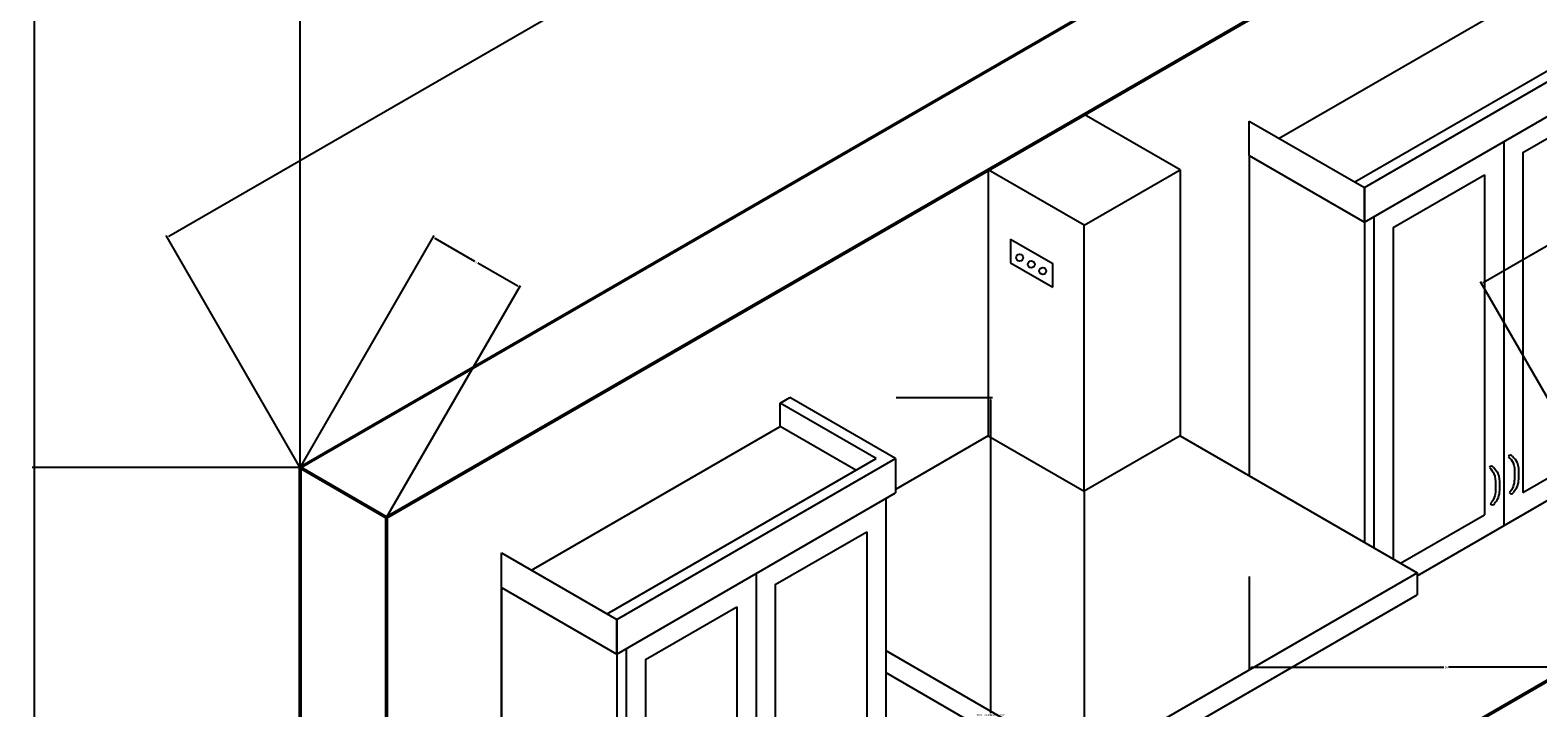
# Model space of a CAD drawing. Units: inches. Extents: x 4150 to 4636, y 2169 to 2592.
# Tile 3 of 8: x 4150 to 4286, y 2438 to 2499. Entities that reach past the tile are written whole.
import ezdxf

# ---------------------------------------------------------------- set-up
doc = ezdxf.new("R2010")
doc.units = ezdxf.units.IN
for name, color, linetype, lineweight in [('A-ANNO-DIMS', 2, 'Continuous', 18), ('A-EQPM', 6, 'Continuous', 25), ('A-FLOR-CASE', 3, 'Continuous', 25), ('A-WALL', 7, 'Continuous', 50)]:
    doc.layers.add(name, color=color, linetype=linetype, lineweight=lineweight)
doc.styles.get("Standard").update_dxf_attribs({"font": 'arial.ttf'})
doc.dimstyles.get("Standard").update_dxf_attribs({"dimtxt": 0.18, "dimasz": 0.18, "dimexe": 0.18, "dimexo": 0.0625, "dimgap": 0.09, "dimtad": 0, "dimtih": 1, "dimtoh": 1, "dimdec": 4, "dimzin": 0, "dimdsep": 46, "dimtxsty": 'Standard', "dimcen": 0.09, "dimadec": 0, "dimazin": 0, "dimtfac": 1, "dimtdec": 4, "dimtofl": 0, "dimtmove": 0, "dimatfit": 3, "dimfxl": 1, "dimtolj": 1, "dimtzin": 0, "dimarcsym": 0})

# ---------------------------------------------------------------- blocks, each defined once
blk = doc.blocks.new('CUBOARD 1')
for p, q in [((4285.13, 2504.76), (4286, 2505.26)), ((4285.13, 2502.65), (4285.13, 2504.76)), ((4293.79, 2499.76), (4285.13, 2504.76)), ((4295.52, 2499.76), (4286, 2505.26)), ((4262.66, 2489.68), (4285.13, 2502.65)), ((4291.96, 2498.71), (4285.13, 2502.65)), ((4269.49, 2485.74), (4293.79, 2499.76)), ((4270.36, 2485.24), (4295.52, 2499.76)), ((4270.36, 2485.24), (4295.52, 2499.76)), ((4295.52, 2499.76), (4295.52, 2496.65)), ((4270.36, 2482.12), (4295.52, 2496.65)), ((4294.66, 2496.15), (4294.66, 2461.49)), ((4284.67, 2488.39), (4292.93, 2493.15)), ((4292.93, 2493.15), (4292.93, 2462.49)), ((4259.97, 2491.24), (4270.36, 2485.24)), ((4259.97, 2488.12), (4259.97, 2491.24)), ((4282.94, 2489.39), (4282.94, 2454.72)), ((4284.67, 2488.39), (4284.67, 2457.72)), ((4259.97, 2488.12), (4270.36, 2482.12)), ((4259.97, 2488.12), (4259.97, 2459.23)), ((4272.96, 2481.62), (4281.21, 2486.39)), ((4281.21, 2486.39), (4281.21, 2455.72)), ((4270.36, 2485.24), (4270.36, 2482.12)), ((4270.36, 2482.12), (4270.36, 2485.24)), ((4270.36, 2482.12), (4270.36, 2453.23)), ((4271.22, 2482.62), (4271.22, 2452.73)), ((4272.96, 2481.62), (4272.96, 2451.73)), ((4284.67, 2457.72), (4292.93, 2462.49)), ((4275.13, 2450.21), (4294.66, 2461.49)), ((4273.63, 2451.35), (4281.21, 2455.72))]:
    blk.add_line(p, q)
for centre, radius, start, end in [((4283.56, 2460.89), 0.201, 29.3135, 156.7087), ((4281.84, 2459.9), 0.201, 29.3135, 156.7087), ((4283.63, 2457.8), 0.198, 207.8897, 338.1325), ((4281.92, 2456.81), 0.198, 207.8897, 338.1325)]:
    blk.add_arc(centre, radius, start, end)
for points in [[(4281.66, 2459.98), (4281.81, 2459.8), (4282.19, 2459.37), (4282.21, 2458.32), (4282.21, 2457.34), (4281.84, 2456.84), (4281.74, 2456.71)], [(4282.02, 2460), (4282.17, 2459.82), (4282.55, 2459.39), (4282.57, 2458.34), (4282.57, 2457.35), (4282.2, 2456.86), (4282.1, 2456.73)], [(4283.37, 2460.97), (4283.53, 2460.79), (4283.91, 2460.36), (4283.93, 2459.31), (4283.92, 2458.33), (4283.56, 2457.83), (4283.46, 2457.7)], [(4283.73, 2460.99), (4283.89, 2460.81), (4284.27, 2460.38), (4284.29, 2459.33), (4284.28, 2458.34), (4283.91, 2457.85), (4283.82, 2457.72)]]:
    blk.add_open_spline(points, degree=3, knots=[0, 0, 0, 0, 0.695815, 1.679053, 3.025679, 3.502598, 3.502598, 3.502598, 3.502598])
blk = doc.blocks.new('CUBOARD 2')
for p, q in [((4217.63, 2465.79), (4218.5, 2466.29)), ((4217.63, 2463.68), (4217.63, 2465.79)), ((4226.29, 2460.79), (4217.63, 2465.79)), ((4228.02, 2460.79), (4218.5, 2466.29)), ((4195.16, 2450.71), (4217.63, 2463.68)), ((4224.46, 2459.74), (4217.63, 2463.68)), ((4201.99, 2446.77), (4226.29, 2460.79)), ((4202.86, 2446.27), (4228.02, 2460.79)), ((4202.86, 2446.27), (4228.02, 2460.79)), ((4228.02, 2460.79), (4228.02, 2457.68)), ((4202.86, 2443.15), (4228.02, 2457.68)), ((4227.16, 2457.18), (4227.16, 2422.52)), ((4217.17, 2449.42), (4225.43, 2454.18)), ((4225.43, 2454.18), (4225.43, 2423.52)), ((4192.47, 2452.27), (4202.86, 2446.27)), ((4192.47, 2449.15), (4192.47, 2452.27)), ((4215.44, 2450.42), (4215.44, 2415.75)), ((4192.47, 2449.15), (4202.86, 2443.15)), ((4192.47, 2449.15), (4192.47, 2415.49)), ((4217.17, 2449.42), (4217.17, 2418.75)), ((4205.46, 2442.65), (4213.71, 2447.42)), ((4213.71, 2447.42), (4213.71, 2416.75)), ((4202.86, 2446.27), (4202.86, 2443.15)), ((4202.86, 2443.15), (4202.86, 2446.27)), ((4203.72, 2443.65), (4203.72, 2408.99)), ((4202.86, 2443.15), (4202.86, 2409.49)), ((4205.46, 2442.65), (4205.46, 2411.99)), ((4217.17, 2418.75), (4225.43, 2423.52)), ((4203.72, 2408.99), (4227.16, 2422.52)), ((4205.46, 2411.99), (4213.71, 2416.75)), ((4203.72, 2408.99), (4192.47, 2415.49))]:
    blk.add_line(p, q)
for centre, radius, start, end in [((4216.06, 2421.92), 0.201, 29.3135, 156.7087), ((4214.34, 2420.93), 0.201, 29.3135, 156.7087), ((4214.42, 2417.84), 0.198, 207.8897, 338.1325), ((4216.13, 2418.83), 0.198, 207.8897, 338.1325)]:
    blk.add_arc(centre, radius, start, end)
for points in [[(4215.87, 2422), (4216.03, 2421.82), (4216.41, 2421.39), (4216.43, 2420.34), (4216.42, 2419.36), (4216.06, 2418.86), (4215.96, 2418.73)], [(4216.23, 2422.02), (4216.39, 2421.84), (4216.77, 2421.41), (4216.79, 2420.36), (4216.78, 2419.38), (4216.41, 2418.88), (4216.32, 2418.75)], [(4214.16, 2421.01), (4214.31, 2420.83), (4214.69, 2420.4), (4214.71, 2419.35), (4214.71, 2418.37), (4214.34, 2417.87), (4214.24, 2417.74)], [(4214.52, 2421.03), (4214.67, 2420.85), (4215.05, 2420.42), (4215.07, 2419.37), (4215.07, 2418.38), (4214.7, 2417.89), (4214.6, 2417.76)]]:
    blk.add_open_spline(points, degree=3, knots=[0, 0, 0, 0, 0.695815, 1.679053, 3.025679, 3.502598, 3.502598, 3.502598, 3.502598])
blk = doc.blocks.new('AIR FRESH')
for p, q in [((4253.73, 2486.84), (4245.07, 2491.84)), ((4236.41, 2486.84), (4236.41, 2462.84)), ((4245.07, 2481.84), (4236.41, 2486.84)), ((4245.07, 2481.84), (4253.73, 2486.84)), ((4253.73, 2486.84), (4253.73, 2462.84)), ((4245.07, 2457.84), (4245.07, 2481.84)), ((4238.41, 2480.59), (4238.41, 2478.46)), ((4238.41, 2480.59), (4242.22, 2478.39)), ((4238.41, 2478.46), (4242.22, 2476.26)), ((4242.22, 2476.26), (4242.22, 2478.39)), ((4236.41, 2462.84), (4228.02, 2457.99)), ((4236.41, 2462.84), (4245.07, 2457.84)), ((4253.73, 2462.84), (4245.07, 2457.84)), ((4253.73, 2462.84), (4275.13, 2450.48)), ((4245.07, 2457.84), (4245.07, 2433.13)), ((4245.07, 2433.13), (4275.13, 2450.48)), ((4275.13, 2450.48), (4275.13, 2448.48)), ((4245.07, 2431.13), (4275.13, 2448.48)), ((4227.16, 2443.47), (4245.07, 2433.13)), ((4227.16, 2441.47), (4245.07, 2431.13)), ((4245.07, 2433.13), (4245.07, 2431.13))]:
    blk.add_line(p, q)
for centre in [(4239.24, 2478.91), (4240.29, 2478.31), (4241.32, 2477.71)]:
    blk.add_circle(centre, 0.313)
blk = doc.blocks.new('*D33')
at = {"layer": 'A-ANNO-DIMS', "color": 0, "lineweight": -2, "transparency": 16777216}
for p, q in [((4259.97, 2450.15), (4259.97, 2441.77)), ((4295.52, 2450.15), (4295.52, 2441.77)), ((4260.15, 2441.95), (4277.53, 2441.95)), ((4295.34, 2441.95), (4277.96, 2441.95))]:
    blk.add_line(p, q, dxfattribs=at)
at = {"layer": 'A-ANNO-DIMS', "color": 0, "transparency": 16777216}
for points in [[(4260.15, 2441.98), (4260.15, 2441.92), (4259.97, 2441.95)], [(4295.34, 2441.98), (4295.34, 2441.92), (4295.52, 2441.95)]]:
    blk.add_solid(points, dxfattribs=at)
at = {"layer": 'Defpoints', "color": 0, "transparency": 16777216}
for p in [(4259.97, 2450.21), (4295.52, 2450.21), (4295.52, 2441.95)]:
    blk.add_point(p, dxfattribs=at)
at = {"layer": 'A-ANNO-DIMS', "color": 0, "transparency": 16777216, "insert": (4277.75, 2441.95), "char_height": 0.18, "attachment_point": 5}
blk.add_mtext('\\A1;36', dxfattribs=at)
blk = doc.blocks.new('*D34')
at = {"layer": 'A-ANNO-DIMS', "color": 0, "lineweight": -2, "transparency": 16777216}
for p, q in [((4228.09, 2466.29), (4236.8, 2466.29)), ((4236.62, 2466.11), (4236.62, 2437.82)), ((4236.62, 2409.17), (4236.62, 2437.46)), ((4228.09, 2408.99), (4236.8, 2408.99))]:
    blk.add_line(p, q, dxfattribs=at)
at = {"layer": 'A-ANNO-DIMS', "color": 0, "transparency": 16777216}
for points in [[(4236.59, 2466.11), (4236.65, 2466.11), (4236.62, 2466.29)], [(4236.59, 2409.17), (4236.65, 2409.17), (4236.62, 2408.99)]]:
    blk.add_solid(points, dxfattribs=at)
at = {"layer": 'Defpoints', "color": 0, "transparency": 16777216}
for p in [(4228.02, 2466.29), (4236.62, 2466.29), (4228.02, 2408.99)]:
    blk.add_point(p, dxfattribs=at)
at = {"layer": 'A-ANNO-DIMS', "color": 0, "transparency": 16777216, "insert": (4236.62, 2437.64), "char_height": 0.18, "attachment_point": 5}
blk.add_mtext('\\A1;WALL CUPBOARD 2 57', dxfattribs=at)
blk = doc.blocks.new('*D36')
at = {"layer": 'A-ANNO-DIMS', "color": 0, "lineweight": -2, "transparency": 16777216}
for p, q in [((4174.28, 2460.03), (4174.28, 2592.15)), ((4174.46, 2591.97), (4402.51, 2591.97)), ((4631.36, 2591.97), (4403.31, 2591.97)), ((4631.54, 2412.03), (4631.54, 2592.15))]:
    blk.add_line(p, q, dxfattribs=at)
at = {"layer": 'A-ANNO-DIMS', "color": 0, "transparency": 16777216}
for points in [[(4174.46, 2592), (4174.46, 2591.94), (4174.28, 2591.97)], [(4631.36, 2592), (4631.36, 2591.94), (4631.54, 2591.97)]]:
    blk.add_solid(points, dxfattribs=at)
at = {"layer": 'Defpoints', "color": 0, "transparency": 16777216}
for p in [(4631.54, 2591.97), (4174.28, 2459.97), (4631.54, 2411.97)]:
    blk.add_point(p, dxfattribs=at)
at = {"layer": 'A-ANNO-DIMS', "color": 0, "transparency": 16777216, "insert": (4402.91, 2591.97), "char_height": 0.18, "attachment_point": 5}
blk.add_mtext('\\A1;457.3', dxfattribs=at)
blk = doc.blocks.new('*D37')
at = {"layer": 'A-ANNO-DIMS', "color": 0, "lineweight": -2, "transparency": 16777216}
for p, q in [((4361.28, 2567.97), (4150.1, 2567.97)), ((4150.28, 2567.79), (4150.28, 2379.06)), ((4150.28, 2189.96), (4150.28, 2378.69)), ((4434.34, 2189.78), (4150.1, 2189.78))]:
    blk.add_line(p, q, dxfattribs=at)
at = {"layer": 'A-ANNO-DIMS', "color": 0, "transparency": 16777216}
for points in [[(4150.25, 2567.79), (4150.31, 2567.79), (4150.28, 2567.97)], [(4150.25, 2189.96), (4150.31, 2189.96), (4150.28, 2189.78)]]:
    blk.add_solid(points, dxfattribs=at)
at = {"layer": 'Defpoints', "color": 0, "transparency": 16777216}
for p in [(4361.34, 2567.97), (4150.28, 2189.78), (4434.4, 2189.78)]:
    blk.add_point(p, dxfattribs=at)
at = {"layer": 'A-ANNO-DIMS', "color": 0, "transparency": 16777216, "insert": (4150.28, 2378.87), "char_height": 0.18, "attachment_point": 5}
blk.add_mtext('\\A1;378.2', dxfattribs=at)
blk = doc.blocks.new('*D41')
at = {"layer": 'A-ANNO-DIMS', "color": 0, "lineweight": -2, "transparency": 16777216}
for p, q in [((4174.22, 2459.97), (4150.1, 2459.97)), ((4150.28, 2459.79), (4150.28, 2404.53)), ((4150.28, 2348.92), (4150.28, 2404.17)), ((4174.22, 2348.74), (4150.1, 2348.74))]:
    blk.add_line(p, q, dxfattribs=at)
at = {"layer": 'A-ANNO-DIMS', "color": 0, "transparency": 16777216}
for points in [[(4150.25, 2459.79), (4150.31, 2459.79), (4150.28, 2459.97)], [(4150.25, 2348.92), (4150.31, 2348.92), (4150.28, 2348.74)]]:
    blk.add_solid(points, dxfattribs=at)
at = {"layer": 'Defpoints', "color": 0, "transparency": 16777216}
for p in [(4174.28, 2459.97), (4150.28, 2348.74), (4174.28, 2348.74)]:
    blk.add_point(p, dxfattribs=at)
at = {"layer": 'A-ANNO-DIMS', "color": 0, "transparency": 16777216, "insert": (4150.28, 2404.35), "char_height": 0.18, "attachment_point": 5}
blk.add_mtext('\\A1;111.23', dxfattribs=at)
blk = doc.blocks.new('*D42')
at = {"layer": 'A-ANNO-DIMS', "color": 0, "lineweight": -2, "transparency": 16777216}
for p, q in [((4349.19, 2588.66), (4256.1, 2534.92)), ((4361.31, 2568.02), (4349.25, 2588.91)), ((4162.44, 2480.84), (4255.52, 2534.58)), ((4174.25, 2460.02), (4162.19, 2480.91))]:
    blk.add_line(p, q, dxfattribs=at)
at = {"layer": 'A-ANNO-DIMS', "color": 0, "transparency": 16777216}
for points in [[(4349.17, 2588.69), (4349.2, 2588.63), (4349.34, 2588.75)], [(4162.42, 2480.87), (4162.45, 2480.81), (4162.28, 2480.75)]]:
    blk.add_solid(points, dxfattribs=at)
at = {"layer": 'Defpoints', "color": 0, "transparency": 16777216}
for p in [(4349.34, 2588.75), (4361.34, 2567.97), (4174.28, 2459.97)]:
    blk.add_point(p, dxfattribs=at)
at = {"layer": 'A-ANNO-DIMS', "color": 0, "transparency": 16777216, "insert": (4255.81, 2534.75), "char_height": 0.18, "attachment_point": 5}
blk.add_mtext('\\A1;216', dxfattribs=at)
blk = doc.blocks.new('*D44')
at = {"layer": 'A-ANNO-DIMS', "color": 0, "lineweight": -2, "transparency": 16777216}
for p, q in [((4174.31, 2460.02), (4186.37, 2480.91)), ((4186.44, 2480.66), (4190.03, 2478.59)), ((4193.92, 2476.34), (4190.33, 2478.41)), ((4182.11, 2455.52), (4194.16, 2476.41))]:
    blk.add_line(p, q, dxfattribs=at)
at = {"layer": 'A-ANNO-DIMS', "color": 0, "transparency": 16777216}
for points in [[(4186.45, 2480.69), (4186.42, 2480.63), (4186.28, 2480.75)], [(4193.93, 2476.37), (4193.9, 2476.31), (4194.07, 2476.25)]]:
    blk.add_solid(points, dxfattribs=at)
at = {"layer": 'Defpoints', "color": 0, "transparency": 16777216}
for p in [(4194.07, 2476.25), (4174.28, 2459.97), (4182.07, 2455.47)]:
    blk.add_point(p, dxfattribs=at)
at = {"layer": 'A-ANNO-DIMS', "color": 0, "transparency": 16777216, "insert": (4190.18, 2478.5), "char_height": 0.18, "attachment_point": 5}
blk.add_mtext('\\A1;9', dxfattribs=at)
blk = doc.blocks.new('*D53')
at = {"layer": 'A-ANNO-DIMS', "color": 0, "lineweight": -2, "transparency": 16777216}
for p, q in [((4315.69, 2496.64), (4298.7, 2486.83)), ((4327.81, 2476), (4315.75, 2496.89)), ((4281.08, 2476.66), (4298.07, 2486.47)), ((4292.89, 2455.84), (4280.84, 2476.73))]:
    blk.add_line(p, q, dxfattribs=at)
at = {"layer": 'A-ANNO-DIMS', "color": 0, "transparency": 16777216}
for points in [[(4315.67, 2496.67), (4315.7, 2496.61), (4315.84, 2496.73)], [(4281.07, 2476.69), (4281.1, 2476.64), (4280.93, 2476.57)]]:
    blk.add_solid(points, dxfattribs=at)
at = {"layer": 'Defpoints', "color": 0, "transparency": 16777216}
for p in [(4315.84, 2496.73), (4327.84, 2475.95), (4292.93, 2455.79)]:
    blk.add_point(p, dxfattribs=at)
at = {"layer": 'A-ANNO-DIMS', "color": 0, "transparency": 16777216, "insert": (4298.38, 2486.65), "char_height": 0.18, "attachment_point": 5}
blk.add_mtext('\\A1;40.32', dxfattribs=at)

msp = doc.modelspace()

# ---------------------------------------------------------------- linework, layer by layer
at = {"layer": 'A-FLOR-CASE'}
msp.add_line((4192.4665, 2415.4873), (4192.4665, 2452.2661), dxfattribs=at)
at = {"layer": 'A-WALL'}
for p, q in [((4182.0742, 2455.4652), (4361.3415, 2558.9652)), ((4174.28, 2459.9652), (4278.203, 2519.9652)), ((4174.28, 2339.9652), (4174.28, 2459.9652)), ((4182.0742, 2455.4652), (4174.28, 2459.9652)), ((4182.0742, 2344.2364), (4182.0742, 2455.4652)), ((4190.7345, 2385.2364), (4289.9267, 2442.5051))]:
    msp.add_line(p, q, dxfattribs=at)

# ---------------------------------------------------------------- block references
at = {"layer": 'A-EQPM'}
msp.add_blockref('AIR FRESH', (0, 0), dxfattribs=at)
at = {"layer": 'A-FLOR-CASE'}
for name in ['CUBOARD 1', 'CUBOARD 2']:
    msp.add_blockref(name, (0, 0), dxfattribs=at)

# ---------------------------------------------------------------- dimensions: what is measured, and where the dimension line sits
at = {"layer": 'A-ANNO-DIMS'}
for base, p1, p2, override, picture, middle in [((4631.5414, 2591.9652), (4174.28, 2459.9652), (4631.5414, 2411.9652), {"dimdec": 1, "dimlfac": 1, "dimrnd": 0, "dimzin": 0, "dimdsep": 46, "dimlunit": 2}, '*D36', (4402.9107, 2591.9652)), ((4295.5235, 2441.9524), (4259.9665, 2450.2105), (4295.5235, 2450.2105), {"dimdec": 0, "dimlfac": 1, "dimrnd": 0, "dimzin": 0, "dimdsep": 46, "dimlunit": 2}, '*D33', (4277.745, 2441.9524))]:
    dim = msp.add_linear_dim(base=base, p1=p1, p2=p2, dimstyle='Standard', override=override, dxfattribs=at)
    dim.commit()
    dim.dimension.update_dxf_attribs({"geometry": picture, "text_midpoint": middle})
for base, p1, p2, angle, override, picture, middle in [((4349.3415, 2588.7498), (4174.28, 2459.9652), (4361.3415, 2567.9652), 30, {"dimdec": 0, "dimlfac": 1, "dimrnd": 0, "dimzin": 0, "dimdsep": 46, "dimlunit": 2}, '*D42', (4255.8107, 2534.7498)), ((4150.28, 2189.7836), (4361.3415, 2567.9652), (4434.4021, 2189.7836), 90, {"dimdec": 1, "dimlfac": 1, "dimrnd": 0, "dimzin": 0, "dimdsep": 46, "dimlunit": 2}, '*D37', (4150.28, 2378.8744)), ((4315.8419, 2496.7305), (4292.9255, 2455.7868), (4327.8419, 2475.9458), 30, {"dimdec": 2, "dimlfac": 1, "dimrnd": 0, "dimzin": 0, "dimdsep": 46, "dimlunit": 2}, '*D53', (4298.3837, 2486.6509)), ((4194.0742, 2476.2498), (4174.28, 2459.9652), (4182.0742, 2455.4652), 330, {"dimdec": 0, "dimlfac": 1, "dimrnd": 0, "dimzin": 0, "dimdsep": 46, "dimlunit": 2}, '*D44', (4190.1771, 2478.4998)), ((4150.28, 2348.7364), (4174.28, 2459.9652), (4174.28, 2348.7364), 90, {"dimdec": 2, "dimlfac": 1, "dimrnd": 0, "dimzin": 0, "dimdsep": 46, "dimlunit": 2}, '*D41', (4150.28, 2404.3508))]:
    dim = msp.add_linear_dim(base=base, p1=p1, p2=p2, angle=angle, dimstyle='Standard', override=override, dxfattribs=at)
    dim.commit()
    dim.dimension.update_dxf_attribs({"geometry": picture, "text_midpoint": middle})
dim = msp.add_linear_dim(base=(4236.6197, 2466.2949), p1=(4228.0235, 2408.9873), p2=(4228.0235, 2466.2949), angle=90, text='WALL CUPBOARD 2 <>', dimstyle='Standard', override={"dimdec": 0, "dimlfac": 1, "dimrnd": 0, "dimzin": 0, "dimdsep": 46, "dimlunit": 2}, dxfattribs=at)
dim.commit()
dim.dimension.update_dxf_attribs({"geometry": '*D34', "text_midpoint": (4236.6197, 2437.6411)})

doc.saveas('drawing.dxf')
